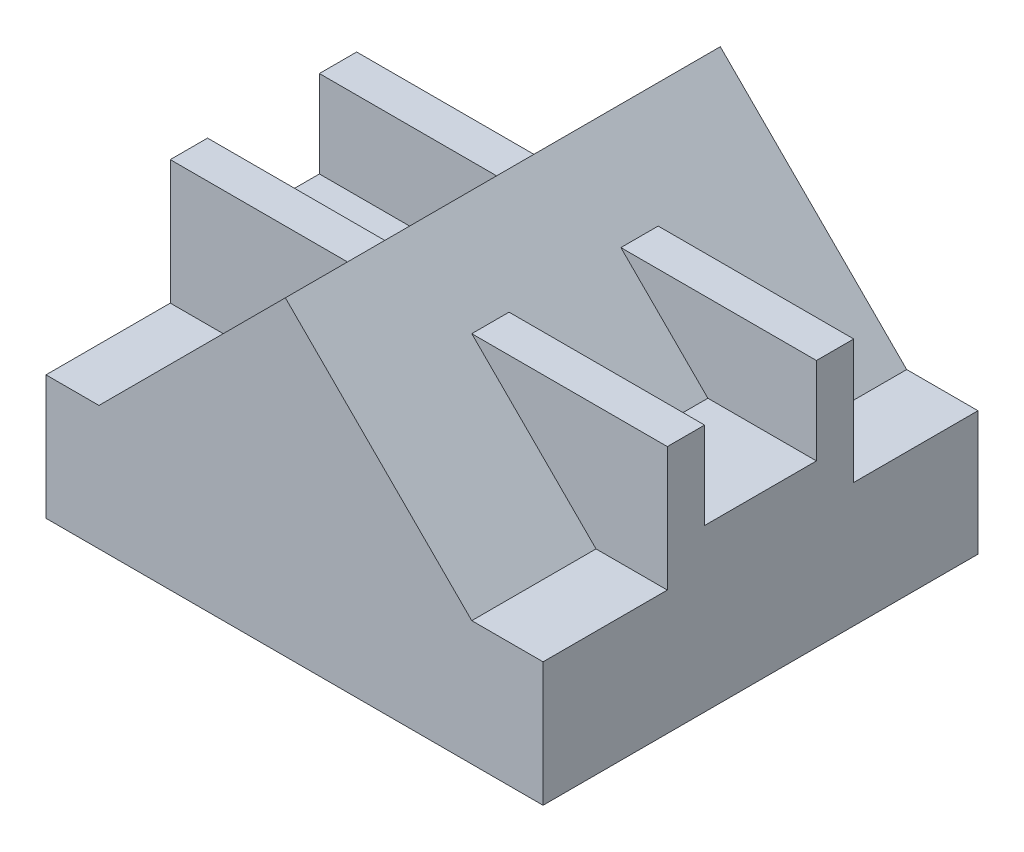
ISO-10303-21;
HEADER;
FILE_DESCRIPTION(('STEP AP214'),'2;1');
FILE_NAME('part.step','',(''),(''),'','','');
FILE_SCHEMA(('AUTOMOTIVE_DESIGN { 1 0 10303 214 1 1 1 1 }'));
ENDSEC;
DATA;
#1=APPLICATION_CONTEXT('core data for automotive mechanical design processes');
#2=APPLICATION_PROTOCOL_DEFINITION('international standard','automotive_design',2000,#1);
#3=PRODUCT_CONTEXT('',#1,'mechanical');
#4=PRODUCT('Part','Part','',(#3));
#5=PRODUCT_RELATED_PRODUCT_CATEGORY('part','',(#4));
#6=PRODUCT_DEFINITION_FORMATION('','',#4);
#7=PRODUCT_DEFINITION_CONTEXT('part definition',#1,'design');
#8=PRODUCT_DEFINITION('design','',#6,#7);
#9=PRODUCT_DEFINITION_SHAPE('','',#8);
#10=(LENGTH_UNIT() NAMED_UNIT(*) SI_UNIT(.MILLI.,.METRE.));
#11=(NAMED_UNIT(*) PLANE_ANGLE_UNIT() SI_UNIT($,.RADIAN.));
#12=(NAMED_UNIT(*) SI_UNIT($,.STERADIAN.) SOLID_ANGLE_UNIT());
#13=UNCERTAINTY_MEASURE_WITH_UNIT(LENGTH_MEASURE(1.E-05),#10,'distance_accuracy_value','');
#14=(GEOMETRIC_REPRESENTATION_CONTEXT(3) GLOBAL_UNCERTAINTY_ASSIGNED_CONTEXT((#13)) GLOBAL_UNIT_ASSIGNED_CONTEXT((#10,
#11,#12)) REPRESENTATION_CONTEXT('',''));
#15=CARTESIAN_POINT('',(0.,0.,0.));
#16=DIRECTION('',(0.,0.,1.));
#17=DIRECTION('',(1.,0.,0.));
#18=AXIS2_PLACEMENT_3D('',#15,#16,#17);
#19=CARTESIAN_POINT('',(75.0000000000014,50.,87.5));
#20=DIRECTION('',(0.,-1.,0.));
#21=DIRECTION('',(0.,0.,-1.));
#22=AXIS2_PLACEMENT_3D('',#19,#20,#21);
#23=PLANE('',#22);
#24=DIRECTION('',(0.,0.,-1.));
#25=VECTOR('',#24,1.);
#26=CARTESIAN_POINT('',(103.688965800971,50.,87.5));
#27=LINE('',#26,#25);
#28=CARTESIAN_POINT('',(103.688965800971,50.,87.5));
#29=VERTEX_POINT('',#28);
#30=CARTESIAN_POINT('',(103.688965800971,50.,37.5));
#31=VERTEX_POINT('',#30);
#32=EDGE_CURVE('E350',#29,#31,#27,.T.);
#33=ORIENTED_EDGE('',*,*,#32,.T.);
#34=DIRECTION('',(1.,0.,0.));
#35=VECTOR('',#34,1.);
#36=CARTESIAN_POINT('',(-96.3110341990287,50.,37.5));
#37=LINE('',#36,#35);
#38=CARTESIAN_POINT('',(75.0000000000014,50.,37.5));
#39=VERTEX_POINT('',#38);
#40=EDGE_CURVE('E255',#39,#31,#37,.T.);
#41=ORIENTED_EDGE('',*,*,#40,.F.);
#42=DIRECTION('',(0.,0.,-1.));
#43=VECTOR('',#42,1.);
#44=CARTESIAN_POINT('',(75.0000000000014,50.,87.5));
#45=LINE('',#44,#43);
#46=CARTESIAN_POINT('',(75.0000000000014,50.,87.5));
#47=VERTEX_POINT('',#46);
#48=EDGE_CURVE('E343',#47,#39,#45,.T.);
#49=ORIENTED_EDGE('',*,*,#48,.F.);
#50=DIRECTION('',(-1.,0.,0.));
#51=VECTOR('',#50,1.);
#52=CARTESIAN_POINT('',(75.0000000000014,50.,87.5));
#53=LINE('',#52,#51);
#54=EDGE_CURVE('E307',#29,#47,#53,.T.);
#55=ORIENTED_EDGE('',*,*,#54,.F.);
#56=EDGE_LOOP('',(#33,#41,#49,#55));
#57=FACE_BOUND('',#56,.T.);
#58=ADVANCED_FACE('F39',(#57),#23,.F.);
#59=CARTESIAN_POINT('',(-96.3110341990287,50.,87.5));
#60=DIRECTION('',(0.,-1.,0.));
#61=DIRECTION('',(0.,0.,-1.));
#62=AXIS2_PLACEMENT_3D('',#59,#60,#61);
#63=PLANE('',#62);
#64=DIRECTION('',(0.,0.,-1.));
#65=VECTOR('',#64,1.);
#66=CARTESIAN_POINT('',(-74.9999999999992,50.,87.5));
#67=LINE('',#66,#65);
#68=CARTESIAN_POINT('',(-74.9999999999992,50.,87.5));
#69=VERTEX_POINT('',#68);
#70=CARTESIAN_POINT('',(-74.9999999999992,50.,37.5));
#71=VERTEX_POINT('',#70);
#72=EDGE_CURVE('E339',#69,#71,#67,.T.);
#73=ORIENTED_EDGE('',*,*,#72,.T.);
#74=CARTESIAN_POINT('',(-96.3110341990287,50.,37.5));
#75=VERTEX_POINT('',#74);
#76=EDGE_CURVE('E253',#75,#71,#37,.T.);
#77=ORIENTED_EDGE('',*,*,#76,.F.);
#78=DIRECTION('',(0.,0.,-1.));
#79=VECTOR('',#78,1.);
#80=CARTESIAN_POINT('',(-96.3110341990287,50.,87.5));
#81=LINE('',#80,#79);
#82=CARTESIAN_POINT('',(-96.3110341990287,50.,87.5));
#83=VERTEX_POINT('',#82);
#84=EDGE_CURVE('E335',#83,#75,#81,.T.);
#85=ORIENTED_EDGE('',*,*,#84,.F.);
#86=DIRECTION('',(-1.,0.,0.));
#87=VECTOR('',#86,1.);
#88=CARTESIAN_POINT('',(-96.3110341990287,50.,87.5));
#89=LINE('',#88,#87);
#90=EDGE_CURVE('E311',#69,#83,#89,.T.);
#91=ORIENTED_EDGE('',*,*,#90,.F.);
#92=EDGE_LOOP('',(#73,#77,#85,#91));
#93=FACE_BOUND('',#92,.T.);
#94=ADVANCED_FACE('F400',(#93),#63,.F.);
#95=CARTESIAN_POINT('',(-96.3110341990287,0.,87.5));
#96=DIRECTION('',(1.,0.,0.));
#97=DIRECTION('',(0.,0.,-1.));
#98=AXIS2_PLACEMENT_3D('',#95,#96,#97);
#99=PLANE('',#98);
#100=DIRECTION('',(0.,-1.,0.));
#101=VECTOR('',#100,1.);
#102=CARTESIAN_POINT('',(-96.3110341990287,0.,-87.5));
#103=LINE('',#102,#101);
#104=CARTESIAN_POINT('',(-96.3110341990287,50.,-87.5));
#105=VERTEX_POINT('',#104);
#106=CARTESIAN_POINT('',(-96.3110341990287,0.,-87.5));
#107=VERTEX_POINT('',#106);
#108=EDGE_CURVE('E300',#105,#107,#103,.T.);
#109=ORIENTED_EDGE('',*,*,#108,.T.);
#110=DIRECTION('',(0.,0.,-1.));
#111=VECTOR('',#110,1.);
#112=CARTESIAN_POINT('',(-96.3110341990287,0.,87.5));
#113=LINE('',#112,#111);
#114=CARTESIAN_POINT('',(-96.3110341990287,0.,87.5));
#115=VERTEX_POINT('',#114);
#116=EDGE_CURVE('E355',#115,#107,#113,.T.);
#117=ORIENTED_EDGE('',*,*,#116,.F.);
#118=DIRECTION('',(0.,-1.,0.));
#119=VECTOR('',#118,1.);
#120=CARTESIAN_POINT('',(-96.3110341990287,0.,87.5));
#121=LINE('',#120,#119);
#122=EDGE_CURVE('E298',#83,#115,#121,.T.);
#123=ORIENTED_EDGE('',*,*,#122,.F.);
#124=ORIENTED_EDGE('',*,*,#84,.T.);
#125=DIRECTION('',(0.,-1.,0.));
#126=VECTOR('',#125,1.);
#127=CARTESIAN_POINT('',(-96.3110341990287,50.,37.5));
#128=LINE('',#127,#126);
#129=CARTESIAN_POINT('',(-96.3110341990287,100.,37.5));
#130=VERTEX_POINT('',#129);
#131=EDGE_CURVE('E235',#130,#75,#128,.T.);
#132=ORIENTED_EDGE('',*,*,#131,.F.);
#133=DIRECTION('',(0.,0.,1.));
#134=VECTOR('',#133,1.);
#135=CARTESIAN_POINT('',(-96.3110341990287,100.,37.5));
#136=LINE('',#135,#134);
#137=CARTESIAN_POINT('',(-96.3110341990287,100.,22.5));
#138=VERTEX_POINT('',#137);
#139=EDGE_CURVE('E228',#138,#130,#136,.T.);
#140=ORIENTED_EDGE('',*,*,#139,.F.);
#141=DIRECTION('',(0.,1.,0.));
#142=VECTOR('',#141,1.);
#143=CARTESIAN_POINT('',(-96.3110341990287,100.,22.5));
#144=LINE('',#143,#142);
#145=CARTESIAN_POINT('',(-96.3110341990287,65.,22.5));
#146=VERTEX_POINT('',#145);
#147=EDGE_CURVE('E229',#146,#138,#144,.T.);
#148=ORIENTED_EDGE('',*,*,#147,.F.);
#149=DIRECTION('',(0.,0.,1.));
#150=VECTOR('',#149,1.);
#151=CARTESIAN_POINT('',(-96.3110341990287,65.,22.5));
#152=LINE('',#151,#150);
#153=CARTESIAN_POINT('',(-96.3110341990287,65.,-22.5));
#154=VERTEX_POINT('',#153);
#155=EDGE_CURVE('E224',#154,#146,#152,.T.);
#156=ORIENTED_EDGE('',*,*,#155,.F.);
#157=DIRECTION('',(0.,-1.,0.));
#158=VECTOR('',#157,1.);
#159=CARTESIAN_POINT('',(-96.3110341990287,65.,-22.5));
#160=LINE('',#159,#158);
#161=CARTESIAN_POINT('',(-96.3110341990287,100.,-22.5));
#162=VERTEX_POINT('',#161);
#163=EDGE_CURVE('E209',#162,#154,#160,.T.);
#164=ORIENTED_EDGE('',*,*,#163,.F.);
#165=DIRECTION('',(0.,0.,1.));
#166=VECTOR('',#165,1.);
#167=CARTESIAN_POINT('',(-96.3110341990287,100.,-22.5));
#168=LINE('',#167,#166);
#169=CARTESIAN_POINT('',(-96.3110341990287,100.,-37.5));
#170=VERTEX_POINT('',#169);
#171=EDGE_CURVE('E196',#170,#162,#168,.T.);
#172=ORIENTED_EDGE('',*,*,#171,.F.);
#173=DIRECTION('',(0.,1.,0.));
#174=VECTOR('',#173,1.);
#175=CARTESIAN_POINT('',(-96.3110341990287,100.,-37.5));
#176=LINE('',#175,#174);
#177=CARTESIAN_POINT('',(-96.3110341990287,50.,-37.5));
#178=VERTEX_POINT('',#177);
#179=EDGE_CURVE('E61',#178,#170,#176,.T.);
#180=ORIENTED_EDGE('',*,*,#179,.F.);
#181=EDGE_CURVE('E312',#178,#105,#81,.T.);
#182=ORIENTED_EDGE('',*,*,#181,.T.);
#183=EDGE_LOOP('',(#109,#117,#123,#124,#132,#140,#148,#156,#164,#172,#180,#182));
#184=FACE_BOUND('',#183,.T.);
#185=ADVANCED_FACE('F41',(#184),#99,.F.);
#186=CARTESIAN_POINT('',(-96.3110341990287,0.,87.5));
#187=DIRECTION('',(0.,1.,0.));
#188=DIRECTION('',(0.,0.,1.));
#189=AXIS2_PLACEMENT_3D('',#186,#187,#188);
#190=PLANE('',#189);
#191=DIRECTION('',(1.,0.,0.));
#192=VECTOR('',#191,1.);
#193=CARTESIAN_POINT('',(-96.3110341990287,0.,-87.5));
#194=LINE('',#193,#192);
#195=CARTESIAN_POINT('',(103.688965800971,0.,-87.5));
#196=VERTEX_POINT('',#195);
#197=EDGE_CURVE('E320',#107,#196,#194,.T.);
#198=ORIENTED_EDGE('',*,*,#197,.T.);
#199=DIRECTION('',(0.,0.,-1.));
#200=VECTOR('',#199,1.);
#201=CARTESIAN_POINT('',(103.688965800971,0.,87.5));
#202=LINE('',#201,#200);
#203=CARTESIAN_POINT('',(103.688965800971,0.,87.5));
#204=VERTEX_POINT('',#203);
#205=EDGE_CURVE('E348',#204,#196,#202,.T.);
#206=ORIENTED_EDGE('',*,*,#205,.F.);
#207=DIRECTION('',(1.,0.,0.));
#208=VECTOR('',#207,1.);
#209=CARTESIAN_POINT('',(-96.3110341990287,0.,87.5));
#210=LINE('',#209,#208);
#211=EDGE_CURVE('E305',#115,#204,#210,.T.);
#212=ORIENTED_EDGE('',*,*,#211,.F.);
#213=ORIENTED_EDGE('',*,*,#116,.T.);
#214=EDGE_LOOP('',(#198,#206,#212,#213));
#215=FACE_BOUND('',#214,.T.);
#216=ADVANCED_FACE('F389',(#215),#190,.F.);
#217=CARTESIAN_POINT('',(103.688965800971,0.,87.5));
#218=DIRECTION('',(-1.,0.,0.));
#219=DIRECTION('',(0.,0.,1.));
#220=AXIS2_PLACEMENT_3D('',#217,#218,#219);
#221=PLANE('',#220);
#222=DIRECTION('',(0.,1.,0.));
#223=VECTOR('',#222,1.);
#224=CARTESIAN_POINT('',(103.688965800971,0.,-87.5));
#225=LINE('',#224,#223);
#226=CARTESIAN_POINT('',(103.688965800971,50.,-87.5));
#227=VERTEX_POINT('',#226);
#228=EDGE_CURVE('E317',#196,#227,#225,.T.);
#229=ORIENTED_EDGE('',*,*,#228,.T.);
#230=CARTESIAN_POINT('',(103.688965800971,50.,-37.5));
#231=VERTEX_POINT('',#230);
#232=EDGE_CURVE('E347',#231,#227,#27,.T.);
#233=ORIENTED_EDGE('',*,*,#232,.F.);
#234=DIRECTION('',(0.,1.,0.));
#235=VECTOR('',#234,1.);
#236=CARTESIAN_POINT('',(103.688965800971,100.,-37.5));
#237=LINE('',#236,#235);
#238=CARTESIAN_POINT('',(103.688965800971,100.,-37.5));
#239=VERTEX_POINT('',#238);
#240=EDGE_CURVE('E234',#231,#239,#237,.T.);
#241=ORIENTED_EDGE('',*,*,#240,.T.);
#242=DIRECTION('',(0.,0.,1.));
#243=VECTOR('',#242,1.);
#244=CARTESIAN_POINT('',(103.688965800971,100.,-22.5));
#245=LINE('',#244,#243);
#246=CARTESIAN_POINT('',(103.688965800971,100.,-22.5));
#247=VERTEX_POINT('',#246);
#248=EDGE_CURVE('E240',#239,#247,#245,.T.);
#249=ORIENTED_EDGE('',*,*,#248,.T.);
#250=DIRECTION('',(0.,-1.,0.));
#251=VECTOR('',#250,1.);
#252=CARTESIAN_POINT('',(103.688965800971,65.,-22.5));
#253=LINE('',#252,#251);
#254=CARTESIAN_POINT('',(103.688965800971,65.,-22.5));
#255=VERTEX_POINT('',#254);
#256=EDGE_CURVE('E238',#247,#255,#253,.T.);
#257=ORIENTED_EDGE('',*,*,#256,.T.);
#258=DIRECTION('',(0.,0.,1.));
#259=VECTOR('',#258,1.);
#260=CARTESIAN_POINT('',(103.688965800971,65.,22.5));
#261=LINE('',#260,#259);
#262=CARTESIAN_POINT('',(103.688965800971,65.,22.5));
#263=VERTEX_POINT('',#262);
#264=EDGE_CURVE('E245',#255,#263,#261,.T.);
#265=ORIENTED_EDGE('',*,*,#264,.T.);
#266=DIRECTION('',(0.,1.,0.));
#267=VECTOR('',#266,1.);
#268=CARTESIAN_POINT('',(103.688965800971,100.,22.5));
#269=LINE('',#268,#267);
#270=CARTESIAN_POINT('',(103.688965800971,100.,22.5));
#271=VERTEX_POINT('',#270);
#272=EDGE_CURVE('E247',#263,#271,#269,.T.);
#273=ORIENTED_EDGE('',*,*,#272,.T.);
#274=DIRECTION('',(0.,0.,1.));
#275=VECTOR('',#274,1.);
#276=CARTESIAN_POINT('',(103.688965800971,100.,37.5));
#277=LINE('',#276,#275);
#278=CARTESIAN_POINT('',(103.688965800971,100.,37.5));
#279=VERTEX_POINT('',#278);
#280=EDGE_CURVE('E218',#271,#279,#277,.T.);
#281=ORIENTED_EDGE('',*,*,#280,.T.);
#282=DIRECTION('',(0.,-1.,0.));
#283=VECTOR('',#282,1.);
#284=CARTESIAN_POINT('',(103.688965800971,50.,37.5));
#285=LINE('',#284,#283);
#286=EDGE_CURVE('E216',#279,#31,#285,.T.);
#287=ORIENTED_EDGE('',*,*,#286,.T.);
#288=ORIENTED_EDGE('',*,*,#32,.F.);
#289=DIRECTION('',(0.,1.,0.));
#290=VECTOR('',#289,1.);
#291=CARTESIAN_POINT('',(103.688965800971,0.,87.5));
#292=LINE('',#291,#290);
#293=EDGE_CURVE('E301',#204,#29,#292,.T.);
#294=ORIENTED_EDGE('',*,*,#293,.F.);
#295=ORIENTED_EDGE('',*,*,#205,.T.);
#296=EDGE_LOOP('',(#229,#233,#241,#249,#257,#265,#273,#281,#287,#288,#294,#295));
#297=FACE_BOUND('',#296,.T.);
#298=ADVANCED_FACE('F413',(#297),#221,.F.);
#299=CARTESIAN_POINT('',(75.0000000000014,50.,-37.5));
#300=VERTEX_POINT('',#299);
#301=CARTESIAN_POINT('',(75.0000000000014,50.,-87.5));
#302=VERTEX_POINT('',#301);
#303=EDGE_CURVE('E345',#300,#302,#45,.T.);
#304=ORIENTED_EDGE('',*,*,#303,.F.);
#305=DIRECTION('',(1.,0.,0.));
#306=VECTOR('',#305,1.);
#307=CARTESIAN_POINT('',(-96.3110341990287,50.,-37.5));
#308=LINE('',#307,#306);
#309=EDGE_CURVE('E53',#300,#231,#308,.T.);
#310=ORIENTED_EDGE('',*,*,#309,.T.);
#311=ORIENTED_EDGE('',*,*,#232,.T.);
#312=DIRECTION('',(-1.,0.,0.));
#313=VECTOR('',#312,1.);
#314=CARTESIAN_POINT('',(75.0000000000014,50.,-87.5));
#315=LINE('',#314,#313);
#316=EDGE_CURVE('E325',#227,#302,#315,.T.);
#317=ORIENTED_EDGE('',*,*,#316,.T.);
#318=EDGE_LOOP('',(#304,#310,#311,#317));
#319=FACE_BOUND('',#318,.T.);
#320=ADVANCED_FACE('F407',(#319),#23,.F.);
#321=CARTESIAN_POINT('',(1.36964885867266E-12,125.,87.5));
#322=DIRECTION('',(-0.707106781186548,-0.707106781186547,0.));
#323=DIRECTION('',(0.707106781186547,-0.707106781186548,0.));
#324=AXIS2_PLACEMENT_3D('',#321,#322,#323);
#325=PLANE('',#324);
#326=ORIENTED_EDGE('',*,*,#48,.T.);
#327=DIRECTION('',(-0.707106781186547,0.707106781186548,0.));
#328=VECTOR('',#327,1.);
#329=CARTESIAN_POINT('',(1.36964885867266E-12,125.,37.5));
#330=LINE('',#329,#328);
#331=CARTESIAN_POINT('',(25.0000000000014,100.,37.5));
#332=VERTEX_POINT('',#331);
#333=EDGE_CURVE('E278',#39,#332,#330,.T.);
#334=ORIENTED_EDGE('',*,*,#333,.T.);
#335=DIRECTION('',(0.,0.,-1.));
#336=VECTOR('',#335,1.);
#337=CARTESIAN_POINT('',(25.0000000000014,100.,87.5));
#338=LINE('',#337,#336);
#339=CARTESIAN_POINT('',(25.0000000000014,100.,22.5));
#340=VERTEX_POINT('',#339);
#341=EDGE_CURVE('E293',#332,#340,#338,.T.);
#342=ORIENTED_EDGE('',*,*,#341,.T.);
#343=DIRECTION('',(0.707106781186547,-0.707106781186548,0.));
#344=VECTOR('',#343,1.);
#345=CARTESIAN_POINT('',(1.36964885867266E-12,125.,22.5));
#346=LINE('',#345,#344);
#347=CARTESIAN_POINT('',(60.0000000000013,65.,22.5));
#348=VERTEX_POINT('',#347);
#349=EDGE_CURVE('E295',#340,#348,#346,.T.);
#350=ORIENTED_EDGE('',*,*,#349,.T.);
#351=DIRECTION('',(0.,0.,-1.));
#352=VECTOR('',#351,1.);
#353=CARTESIAN_POINT('',(60.0000000000014,65.,87.5));
#354=LINE('',#353,#352);
#355=CARTESIAN_POINT('',(60.0000000000014,65.,-22.5));
#356=VERTEX_POINT('',#355);
#357=EDGE_CURVE('E289',#348,#356,#354,.T.);
#358=ORIENTED_EDGE('',*,*,#357,.T.);
#359=DIRECTION('',(-0.707106781186547,0.707106781186548,0.));
#360=VECTOR('',#359,1.);
#361=CARTESIAN_POINT('',(1.36419687060531E-12,125.,-22.5));
#362=LINE('',#361,#360);
#363=CARTESIAN_POINT('',(25.0000000000014,100.,-22.5));
#364=VERTEX_POINT('',#363);
#365=EDGE_CURVE('E287',#356,#364,#362,.T.);
#366=ORIENTED_EDGE('',*,*,#365,.T.);
#367=DIRECTION('',(0.,0.,-1.));
#368=VECTOR('',#367,1.);
#369=CARTESIAN_POINT('',(25.0000000000013,100.,87.5));
#370=LINE('',#369,#368);
#371=CARTESIAN_POINT('',(25.0000000000014,100.,-37.5));
#372=VERTEX_POINT('',#371);
#373=EDGE_CURVE('E285',#364,#372,#370,.T.);
#374=ORIENTED_EDGE('',*,*,#373,.T.);
#375=DIRECTION('',(0.707106781186547,-0.707106781186548,0.));
#376=VECTOR('',#375,1.);
#377=CARTESIAN_POINT('',(1.36097524129278E-12,125.,-37.5));
#378=LINE('',#377,#376);
#379=EDGE_CURVE('E274',#372,#300,#378,.T.);
#380=ORIENTED_EDGE('',*,*,#379,.T.);
#381=ORIENTED_EDGE('',*,*,#303,.T.);
#382=DIRECTION('',(-0.707106781186547,0.707106781186548,0.));
#383=VECTOR('',#382,1.);
#384=CARTESIAN_POINT('',(1.36964885867266E-12,125.,-87.5));
#385=LINE('',#384,#383);
#386=CARTESIAN_POINT('',(1.36964885867266E-12,125.,-87.5));
#387=VERTEX_POINT('',#386);
#388=EDGE_CURVE('E324',#302,#387,#385,.T.);
#389=ORIENTED_EDGE('',*,*,#388,.T.);
#390=DIRECTION('',(0.,0.,-1.));
#391=VECTOR('',#390,1.);
#392=CARTESIAN_POINT('',(1.36964885867266E-12,125.,87.5));
#393=LINE('',#392,#391);
#394=CARTESIAN_POINT('',(1.36964885867266E-12,125.,87.5));
#395=VERTEX_POINT('',#394);
#396=EDGE_CURVE('E338',#395,#387,#393,.T.);
#397=ORIENTED_EDGE('',*,*,#396,.F.);
#398=DIRECTION('',(-0.707106781186547,0.707106781186548,0.));
#399=VECTOR('',#398,1.);
#400=CARTESIAN_POINT('',(1.36964885867266E-12,125.,87.5));
#401=LINE('',#400,#399);
#402=EDGE_CURVE('E310',#47,#395,#401,.T.);
#403=ORIENTED_EDGE('',*,*,#402,.F.);
#404=EDGE_LOOP('',(#326,#334,#342,#350,#358,#366,#374,#380,#381,#389,#397,#403));
#405=FACE_BOUND('',#404,.T.);
#406=ADVANCED_FACE('F406',(#405),#325,.F.);
#407=CARTESIAN_POINT('',(1.36964885867266E-12,125.,87.5));
#408=DIRECTION('',(0.707106781186545,-0.70710678118655,0.));
#409=DIRECTION('',(0.70710678118655,0.707106781186545,0.));
#410=AXIS2_PLACEMENT_3D('',#407,#408,#409);
#411=PLANE('',#410);
#412=DIRECTION('',(0.,0.,1.));
#413=VECTOR('',#412,1.);
#414=CARTESIAN_POINT('',(-24.9999999999988,100.,87.5));
#415=LINE('',#414,#413);
#416=CARTESIAN_POINT('',(-24.9999999999988,100.,22.5));
#417=VERTEX_POINT('',#416);
#418=CARTESIAN_POINT('',(-24.9999999999989,100.,37.5));
#419=VERTEX_POINT('',#418);
#420=EDGE_CURVE('E11',#417,#419,#415,.T.);
#421=ORIENTED_EDGE('',*,*,#420,.T.);
#422=DIRECTION('',(-0.70710678118655,-0.707106781186545,0.));
#423=VECTOR('',#422,1.);
#424=CARTESIAN_POINT('',(1.36964885867266E-12,125.,37.5));
#425=LINE('',#424,#423);
#426=EDGE_CURVE('E280',#419,#71,#425,.T.);
#427=ORIENTED_EDGE('',*,*,#426,.T.);
#428=ORIENTED_EDGE('',*,*,#72,.F.);
#429=DIRECTION('',(-0.70710678118655,-0.707106781186545,0.));
#430=VECTOR('',#429,1.);
#431=CARTESIAN_POINT('',(1.36964885867266E-12,125.,87.5));
#432=LINE('',#431,#430);
#433=EDGE_CURVE('E313',#395,#69,#432,.T.);
#434=ORIENTED_EDGE('',*,*,#433,.F.);
#435=ORIENTED_EDGE('',*,*,#396,.T.);
#436=DIRECTION('',(-0.70710678118655,-0.707106781186545,0.));
#437=VECTOR('',#436,1.);
#438=CARTESIAN_POINT('',(1.36964885867266E-12,125.,-87.5));
#439=LINE('',#438,#437);
#440=CARTESIAN_POINT('',(-74.9999999999992,50.,-87.5));
#441=VERTEX_POINT('',#440);
#442=EDGE_CURVE('E330',#387,#441,#439,.T.);
#443=ORIENTED_EDGE('',*,*,#442,.T.);
#444=CARTESIAN_POINT('',(-74.9999999999992,50.,-37.5));
#445=VERTEX_POINT('',#444);
#446=EDGE_CURVE('E333',#445,#441,#67,.T.);
#447=ORIENTED_EDGE('',*,*,#446,.F.);
#448=DIRECTION('',(0.70710678118655,0.707106781186545,0.));
#449=VECTOR('',#448,1.);
#450=CARTESIAN_POINT('',(1.37832247605255E-12,125.,-37.5));
#451=LINE('',#450,#449);
#452=CARTESIAN_POINT('',(-24.9999999999988,100.,-37.5));
#453=VERTEX_POINT('',#452);
#454=EDGE_CURVE('E251',#445,#453,#451,.T.);
#455=ORIENTED_EDGE('',*,*,#454,.T.);
#456=DIRECTION('',(0.,0.,1.));
#457=VECTOR('',#456,1.);
#458=CARTESIAN_POINT('',(-24.9999999999987,100.,87.5));
#459=LINE('',#458,#457);
#460=CARTESIAN_POINT('',(-24.9999999999989,100.,-22.5));
#461=VERTEX_POINT('',#460);
#462=EDGE_CURVE('E199',#453,#461,#459,.T.);
#463=ORIENTED_EDGE('',*,*,#462,.T.);
#464=DIRECTION('',(-0.70710678118655,-0.707106781186545,0.));
#465=VECTOR('',#464,1.);
#466=CARTESIAN_POINT('',(1.37510084674002E-12,125.,-22.5));
#467=LINE('',#466,#465);
#468=CARTESIAN_POINT('',(-59.9999999999991,65.,-22.5));
#469=VERTEX_POINT('',#468);
#470=EDGE_CURVE('E360',#461,#469,#467,.T.);
#471=ORIENTED_EDGE('',*,*,#470,.T.);
#472=DIRECTION('',(0.,0.,1.));
#473=VECTOR('',#472,1.);
#474=CARTESIAN_POINT('',(-59.9999999999991,65.,87.5));
#475=LINE('',#474,#473);
#476=CARTESIAN_POINT('',(-59.9999999999991,65.,22.5));
#477=VERTEX_POINT('',#476);
#478=EDGE_CURVE('E356',#469,#477,#475,.T.);
#479=ORIENTED_EDGE('',*,*,#478,.T.);
#480=DIRECTION('',(0.70710678118655,0.707106781186545,0.));
#481=VECTOR('',#480,1.);
#482=CARTESIAN_POINT('',(1.36964885867266E-12,125.,22.5));
#483=LINE('',#482,#481);
#484=EDGE_CURVE('E50',#477,#417,#483,.T.);
#485=ORIENTED_EDGE('',*,*,#484,.T.);
#486=EDGE_LOOP('',(#421,#427,#428,#434,#435,#443,#447,#455,#463,#471,#479,#485));
#487=FACE_BOUND('',#486,.T.);
#488=ADVANCED_FACE('F365',(#487),#411,.F.);
#489=ORIENTED_EDGE('',*,*,#181,.F.);
#490=EDGE_CURVE('E212',#178,#445,#308,.T.);
#491=ORIENTED_EDGE('',*,*,#490,.T.);
#492=ORIENTED_EDGE('',*,*,#446,.T.);
#493=DIRECTION('',(-1.,0.,0.));
#494=VECTOR('',#493,1.);
#495=CARTESIAN_POINT('',(-96.3110341990287,50.,-87.5));
#496=LINE('',#495,#494);
#497=EDGE_CURVE('E303',#441,#105,#496,.T.);
#498=ORIENTED_EDGE('',*,*,#497,.T.);
#499=EDGE_LOOP('',(#489,#491,#492,#498));
#500=FACE_BOUND('',#499,.T.);
#501=ADVANCED_FACE('F374',(#500),#63,.F.);
#502=CARTESIAN_POINT('',(0.,0.,87.5));
#503=DIRECTION('',(0.,0.,-1.));
#504=DIRECTION('',(-1.,0.,0.));
#505=AXIS2_PLACEMENT_3D('',#502,#503,#504);
#506=PLANE('',#505);
#507=ORIENTED_EDGE('',*,*,#433,.T.);
#508=ORIENTED_EDGE('',*,*,#90,.T.);
#509=ORIENTED_EDGE('',*,*,#122,.T.);
#510=ORIENTED_EDGE('',*,*,#211,.T.);
#511=ORIENTED_EDGE('',*,*,#293,.T.);
#512=ORIENTED_EDGE('',*,*,#54,.T.);
#513=ORIENTED_EDGE('',*,*,#402,.T.);
#514=EDGE_LOOP('',(#507,#508,#509,#510,#511,#512,#513));
#515=FACE_BOUND('',#514,.T.);
#516=ADVANCED_FACE('F394',(#515),#506,.F.);
#517=CARTESIAN_POINT('',(0.,0.,-87.5));
#518=DIRECTION('',(0.,0.,-1.));
#519=DIRECTION('',(-1.,0.,0.));
#520=AXIS2_PLACEMENT_3D('',#517,#518,#519);
#521=PLANE('',#520);
#522=ORIENTED_EDGE('',*,*,#388,.F.);
#523=ORIENTED_EDGE('',*,*,#316,.F.);
#524=ORIENTED_EDGE('',*,*,#228,.F.);
#525=ORIENTED_EDGE('',*,*,#197,.F.);
#526=ORIENTED_EDGE('',*,*,#108,.F.);
#527=ORIENTED_EDGE('',*,*,#497,.F.);
#528=ORIENTED_EDGE('',*,*,#442,.F.);
#529=EDGE_LOOP('',(#522,#523,#524,#525,#526,#527,#528));
#530=FACE_BOUND('',#529,.T.);
#531=ADVANCED_FACE('F385',(#530),#521,.T.);
#532=CARTESIAN_POINT('',(-96.3110341990287,100.,-37.5));
#533=DIRECTION('',(0.,0.,-1.));
#534=DIRECTION('',(0.,1.,0.));
#535=AXIS2_PLACEMENT_3D('',#532,#533,#534);
#536=PLANE('',#535);
#537=ORIENTED_EDGE('',*,*,#454,.F.);
#538=ORIENTED_EDGE('',*,*,#490,.F.);
#539=ORIENTED_EDGE('',*,*,#179,.T.);
#540=DIRECTION('',(1.,0.,0.));
#541=VECTOR('',#540,1.);
#542=CARTESIAN_POINT('',(-96.3110341990287,100.,-37.5));
#543=LINE('',#542,#541);
#544=EDGE_CURVE('E191',#170,#453,#543,.T.);
#545=ORIENTED_EDGE('',*,*,#544,.T.);
#546=EDGE_LOOP('',(#537,#538,#539,#545));
#547=FACE_BOUND('',#546,.T.);
#548=ADVANCED_FACE('F215',(#547),#536,.T.);
#549=CARTESIAN_POINT('',(-96.3110341990287,50.,37.5));
#550=DIRECTION('',(0.,0.,1.));
#551=DIRECTION('',(1.,0.,0.));
#552=AXIS2_PLACEMENT_3D('',#549,#550,#551);
#553=PLANE('',#552);
#554=ORIENTED_EDGE('',*,*,#426,.F.);
#555=DIRECTION('',(1.,0.,0.));
#556=VECTOR('',#555,1.);
#557=CARTESIAN_POINT('',(-96.3110341990287,100.,37.5));
#558=LINE('',#557,#556);
#559=EDGE_CURVE('E254',#130,#419,#558,.T.);
#560=ORIENTED_EDGE('',*,*,#559,.F.);
#561=ORIENTED_EDGE('',*,*,#131,.T.);
#562=ORIENTED_EDGE('',*,*,#76,.T.);
#563=EDGE_LOOP('',(#554,#560,#561,#562));
#564=FACE_BOUND('',#563,.T.);
#565=ADVANCED_FACE('F396',(#564),#553,.T.);
#566=CARTESIAN_POINT('',(-96.3110341990287,100.,-22.5));
#567=DIRECTION('',(0.,1.,0.));
#568=DIRECTION('',(0.,0.,1.));
#569=AXIS2_PLACEMENT_3D('',#566,#567,#568);
#570=PLANE('',#569);
#571=ORIENTED_EDGE('',*,*,#462,.F.);
#572=ORIENTED_EDGE('',*,*,#544,.F.);
#573=ORIENTED_EDGE('',*,*,#171,.T.);
#574=DIRECTION('',(1.,0.,0.));
#575=VECTOR('',#574,1.);
#576=CARTESIAN_POINT('',(-96.3110341990287,100.,-22.5));
#577=LINE('',#576,#575);
#578=EDGE_CURVE('E271',#162,#461,#577,.T.);
#579=ORIENTED_EDGE('',*,*,#578,.T.);
#580=EDGE_LOOP('',(#571,#572,#573,#579));
#581=FACE_BOUND('',#580,.T.);
#582=ADVANCED_FACE('F198',(#581),#570,.T.);
#583=CARTESIAN_POINT('',(-96.3110341990287,65.,-22.5));
#584=DIRECTION('',(0.,0.,1.));
#585=DIRECTION('',(0.,-1.,0.));
#586=AXIS2_PLACEMENT_3D('',#583,#584,#585);
#587=PLANE('',#586);
#588=ORIENTED_EDGE('',*,*,#470,.F.);
#589=ORIENTED_EDGE('',*,*,#578,.F.);
#590=ORIENTED_EDGE('',*,*,#163,.T.);
#591=DIRECTION('',(1.,0.,0.));
#592=VECTOR('',#591,1.);
#593=CARTESIAN_POINT('',(-96.3110341990287,65.,-22.5));
#594=LINE('',#593,#592);
#595=EDGE_CURVE('E270',#154,#469,#594,.T.);
#596=ORIENTED_EDGE('',*,*,#595,.T.);
#597=EDGE_LOOP('',(#588,#589,#590,#596));
#598=FACE_BOUND('',#597,.T.);
#599=ADVANCED_FACE('F375',(#598),#587,.T.);
#600=CARTESIAN_POINT('',(-96.3110341990287,65.,22.5));
#601=DIRECTION('',(0.,1.,0.));
#602=DIRECTION('',(0.,0.,1.));
#603=AXIS2_PLACEMENT_3D('',#600,#601,#602);
#604=PLANE('',#603);
#605=ORIENTED_EDGE('',*,*,#478,.F.);
#606=ORIENTED_EDGE('',*,*,#595,.F.);
#607=ORIENTED_EDGE('',*,*,#155,.T.);
#608=DIRECTION('',(1.,0.,0.));
#609=VECTOR('',#608,1.);
#610=CARTESIAN_POINT('',(-96.3110341990287,65.,22.5));
#611=LINE('',#610,#609);
#612=EDGE_CURVE('E263',#146,#477,#611,.T.);
#613=ORIENTED_EDGE('',*,*,#612,.T.);
#614=EDGE_LOOP('',(#605,#606,#607,#613));
#615=FACE_BOUND('',#614,.T.);
#616=ADVANCED_FACE('F369',(#615),#604,.T.);
#617=CARTESIAN_POINT('',(-96.3110341990287,100.,22.5));
#618=DIRECTION('',(0.,0.,-1.));
#619=DIRECTION('',(-1.,0.,0.));
#620=AXIS2_PLACEMENT_3D('',#617,#618,#619);
#621=PLANE('',#620);
#622=ORIENTED_EDGE('',*,*,#484,.F.);
#623=ORIENTED_EDGE('',*,*,#612,.F.);
#624=ORIENTED_EDGE('',*,*,#147,.T.);
#625=DIRECTION('',(1.,0.,0.));
#626=VECTOR('',#625,1.);
#627=CARTESIAN_POINT('',(-96.3110341990287,100.,22.5));
#628=LINE('',#627,#626);
#629=EDGE_CURVE('E259',#138,#417,#628,.T.);
#630=ORIENTED_EDGE('',*,*,#629,.T.);
#631=EDGE_LOOP('',(#622,#623,#624,#630));
#632=FACE_BOUND('',#631,.T.);
#633=ADVANCED_FACE('F368',(#632),#621,.T.);
#634=CARTESIAN_POINT('',(-96.3110341990287,100.,37.5));
#635=DIRECTION('',(0.,1.,0.));
#636=DIRECTION('',(0.,0.,1.));
#637=AXIS2_PLACEMENT_3D('',#634,#635,#636);
#638=PLANE('',#637);
#639=ORIENTED_EDGE('',*,*,#420,.F.);
#640=ORIENTED_EDGE('',*,*,#629,.F.);
#641=ORIENTED_EDGE('',*,*,#139,.T.);
#642=ORIENTED_EDGE('',*,*,#559,.T.);
#643=EDGE_LOOP('',(#639,#640,#641,#642));
#644=FACE_BOUND('',#643,.T.);
#645=ADVANCED_FACE('F521',(#644),#638,.T.);
#646=ORIENTED_EDGE('',*,*,#341,.F.);
#647=EDGE_CURVE('E256',#332,#279,#558,.T.);
#648=ORIENTED_EDGE('',*,*,#647,.T.);
#649=ORIENTED_EDGE('',*,*,#280,.F.);
#650=EDGE_CURVE('E265',#340,#271,#628,.T.);
#651=ORIENTED_EDGE('',*,*,#650,.F.);
#652=EDGE_LOOP('',(#646,#648,#649,#651));
#653=FACE_BOUND('',#652,.T.);
#654=ADVANCED_FACE('F421',(#653),#638,.T.);
#655=ORIENTED_EDGE('',*,*,#349,.F.);
#656=ORIENTED_EDGE('',*,*,#650,.T.);
#657=ORIENTED_EDGE('',*,*,#272,.F.);
#658=EDGE_CURVE('E266',#348,#263,#611,.T.);
#659=ORIENTED_EDGE('',*,*,#658,.F.);
#660=EDGE_LOOP('',(#655,#656,#657,#659));
#661=FACE_BOUND('',#660,.T.);
#662=ADVANCED_FACE('F430',(#661),#621,.T.);
#663=ORIENTED_EDGE('',*,*,#357,.F.);
#664=ORIENTED_EDGE('',*,*,#658,.T.);
#665=ORIENTED_EDGE('',*,*,#264,.F.);
#666=EDGE_CURVE('E269',#356,#255,#594,.T.);
#667=ORIENTED_EDGE('',*,*,#666,.F.);
#668=EDGE_LOOP('',(#663,#664,#665,#667));
#669=FACE_BOUND('',#668,.T.);
#670=ADVANCED_FACE('F431',(#669),#604,.T.);
#671=ORIENTED_EDGE('',*,*,#365,.F.);
#672=ORIENTED_EDGE('',*,*,#666,.T.);
#673=ORIENTED_EDGE('',*,*,#256,.F.);
#674=EDGE_CURVE('E201',#364,#247,#577,.T.);
#675=ORIENTED_EDGE('',*,*,#674,.F.);
#676=EDGE_LOOP('',(#671,#672,#673,#675));
#677=FACE_BOUND('',#676,.T.);
#678=ADVANCED_FACE('F434',(#677),#587,.T.);
#679=ORIENTED_EDGE('',*,*,#373,.F.);
#680=ORIENTED_EDGE('',*,*,#674,.T.);
#681=ORIENTED_EDGE('',*,*,#248,.F.);
#682=EDGE_CURVE('E204',#372,#239,#543,.T.);
#683=ORIENTED_EDGE('',*,*,#682,.F.);
#684=EDGE_LOOP('',(#679,#680,#681,#683));
#685=FACE_BOUND('',#684,.T.);
#686=ADVANCED_FACE('F438',(#685),#570,.T.);
#687=ORIENTED_EDGE('',*,*,#333,.F.);
#688=ORIENTED_EDGE('',*,*,#40,.T.);
#689=ORIENTED_EDGE('',*,*,#286,.F.);
#690=ORIENTED_EDGE('',*,*,#647,.F.);
#691=EDGE_LOOP('',(#687,#688,#689,#690));
#692=FACE_BOUND('',#691,.T.);
#693=ADVANCED_FACE('F419',(#692),#553,.T.);
#694=ORIENTED_EDGE('',*,*,#379,.F.);
#695=ORIENTED_EDGE('',*,*,#682,.T.);
#696=ORIENTED_EDGE('',*,*,#240,.F.);
#697=ORIENTED_EDGE('',*,*,#309,.F.);
#698=EDGE_LOOP('',(#694,#695,#696,#697));
#699=FACE_BOUND('',#698,.T.);
#700=ADVANCED_FACE('F442',(#699),#536,.T.);
#701=CLOSED_SHELL('',(#58,#94,#185,#216,#298,#320,#406,#488,#501,#516,#531,#548,#565,#582,#599,
#616,#633,#645,#654,#662,#670,#678,#686,#693,#700));
#702=MANIFOLD_SOLID_BREP('B2',#701);
#703=ADVANCED_BREP_SHAPE_REPRESENTATION('',(#18,#702),#14);
#704=SHAPE_DEFINITION_REPRESENTATION(#9,#703);
ENDSEC;
END-ISO-10303-21;
